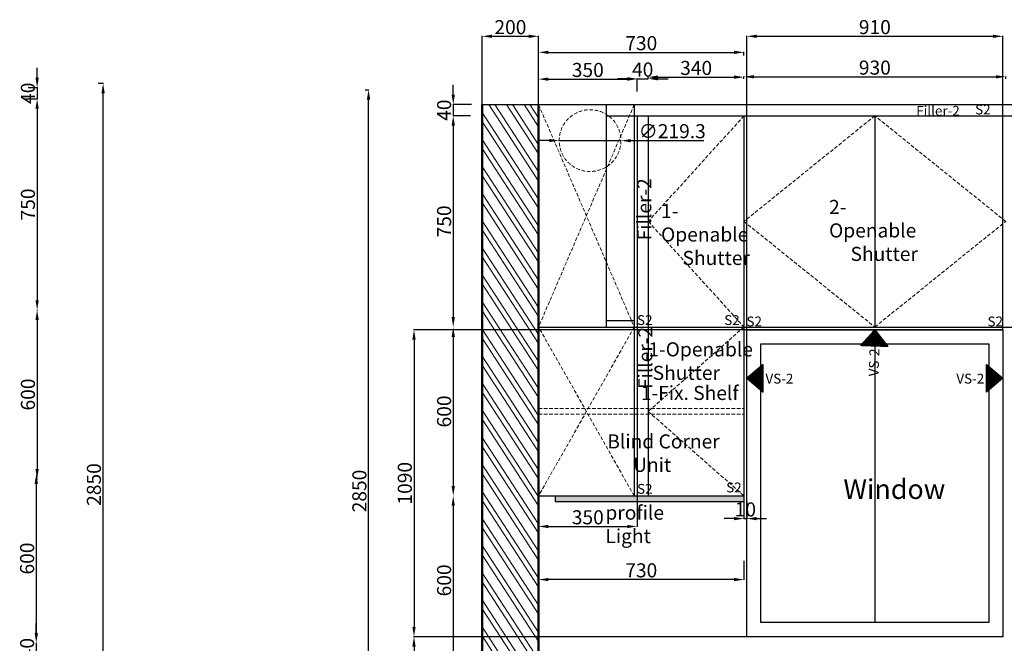
# Model space of a CAD drawing. Units: millimetres. Extents: x 407065 to 421840, y 1168257 to 1177792.
# Tile 16 of 17: x 415758 to 419256, y 1175003 to 1177218. Entities that reach past the tile are written whole.
import ezdxf

# ---------------------------------------------------------------- set-up
doc = ezdxf.new("R2010")
doc.units = ezdxf.units.MM
doc.linetypes.add('DASHED', pattern=[19.05, 12.7, -6.35])
for name, color, linetype, lineweight in [('A-ANNO-DIMS', 6, 'Continuous', 18), ('A-ANNO-TEXT', 30, 'Continuous', 18), ('A-FURN', 3, 'Continuous', 25), ('A-FURN-HIDN', 7, 'DASHED', 18), ('A-FURN-PATT', 252, 'Continuous', 13), ('A-GLAZ', 4, 'Continuous', 25), ('A-WALL', 7, 'Continuous', 50), ('A-WALL-PATT', 8, 'Continuous', 13)]:
    doc.layers.add(name, color=color, linetype=linetype, lineweight=lineweight)
doc.styles.get("Standard").update_dxf_attribs({"font": 'arial.ttf'})
doc.dimstyles.new('ISO-25', dxfattribs={"dimtxt": 50, "dimasz": 35, "dimexe": 1.25, "dimexo": 0.625, "dimtad": 1, "dimdec": 1, "dimtxsty": 'Standard', "dimcen": 35, "dimadec": 0, "dimazin": 0, "dimtfac": 1, "dimtdec": 1, "dimtmove": 0, "dimatfit": 3, "dimfxl": 1, "dimarcsym": 0})

# ---------------------------------------------------------------- blocks, each defined once
blk = doc.blocks.new('*D63')
at = {"layer": 'A-ANNO-DIMS', "color": 0, "lineweight": -2, "transparency": 16777216}
for p, q in [((415819.6, 1177011.4), (415819.6, 1177046.4)), ((415788, 1176976.4), (415820.8, 1176976.4)), ((415819.6, 1176976.4), (415819.6, 1176936.4)), ((415777.3, 1176936.4), (415820.8, 1176936.4)), ((415819.6, 1176901.4), (415819.6, 1176866.4))]:
    blk.add_line(p, q, dxfattribs=at)
at = {"layer": 'A-ANNO-DIMS', "color": 0, "transparency": 16777216}
for points in [[(415813.7, 1177011.4), (415825.4, 1177011.4), (415819.6, 1176976.4)], [(415813.7, 1176901.4), (415825.4, 1176901.4), (415819.6, 1176936.4)]]:
    blk.add_solid(points, dxfattribs=at)
at = {"layer": 'Defpoints', "color": 0, "transparency": 16777216}
for p in [(415787.4, 1176976.4), (415776.6, 1176936.4), (415819.6, 1176936.4)]:
    blk.add_point(p, dxfattribs=at)
at = {"layer": 'A-ANNO-DIMS', "color": 0, "transparency": 16777216, "insert": (415793.4, 1176956.4), "char_height": 50, "attachment_point": 5, "rotation": 90}
blk.add_mtext('40', dxfattribs=at)
blk = doc.blocks.new('*D64')
at = {"layer": 'A-ANNO-DIMS', "color": 0, "lineweight": -2, "transparency": 16777216}
for p, q in [((415820.2, 1176936.4), (415820.8, 1176936.4)), ((415819.6, 1176901.4), (415819.6, 1176221.4)), ((415820.2, 1176186.4), (415820.8, 1176186.4))]:
    blk.add_line(p, q, dxfattribs=at)
at = {"layer": 'A-ANNO-DIMS', "color": 0, "transparency": 16777216}
for points in [[(415813.7, 1176901.4), (415825.4, 1176901.4), (415819.6, 1176936.4)], [(415813.7, 1176221.4), (415825.4, 1176221.4), (415819.6, 1176186.4)]]:
    blk.add_solid(points, dxfattribs=at)
at = {"layer": 'Defpoints', "color": 0, "transparency": 16777216}
for p in [(415819.6, 1176936.4), (415819.6, 1176186.4), (415819.6, 1176186.4)]:
    blk.add_point(p, dxfattribs=at)
at = {"layer": 'A-ANNO-DIMS', "color": 0, "transparency": 16777216, "insert": (415793.4, 1176561.4), "char_height": 50, "attachment_point": 5, "rotation": 90}
blk.add_mtext('750', dxfattribs=at)
blk = doc.blocks.new('*D65')
at = {"layer": 'A-ANNO-DIMS', "color": 0, "lineweight": -2, "transparency": 16777216}
for p, q in [((415818.9, 1176186.4), (415820.8, 1176186.4)), ((415819.6, 1176151.4), (415819.6, 1175621.4)), ((415818.9, 1175586.4), (415820.8, 1175586.4))]:
    blk.add_line(p, q, dxfattribs=at)
at = {"layer": 'A-ANNO-DIMS', "color": 0, "transparency": 16777216}
for points in [[(415813.7, 1176151.4), (415825.4, 1176151.4), (415819.6, 1176186.4)], [(415813.7, 1175621.4), (415825.4, 1175621.4), (415819.6, 1175586.4)]]:
    blk.add_solid(points, dxfattribs=at)
at = {"layer": 'Defpoints', "color": 0, "transparency": 16777216}
for p in [(415818.3, 1176186.4), (415818.3, 1175586.4), (415819.6, 1175586.4)]:
    blk.add_point(p, dxfattribs=at)
at = {"layer": 'A-ANNO-DIMS', "color": 0, "transparency": 16777216, "insert": (415793.4, 1175886.4), "char_height": 50, "attachment_point": 5, "rotation": 90}
blk.add_mtext('600', dxfattribs=at)
blk = doc.blocks.new('*D66')
at = {"layer": 'A-ANNO-DIMS', "color": 0, "lineweight": -2, "transparency": 16777216}
for p, q in [((415817.3, 1175603.9), (415817.9, 1175603.9)), ((415816.7, 1175568.9), (415816.7, 1175038.9)), ((415817.3, 1175003.9), (415817.9, 1175003.9))]:
    blk.add_line(p, q, dxfattribs=at)
at = {"layer": 'A-ANNO-DIMS', "color": 0, "transparency": 16777216}
for points in [[(415810.8, 1175568.9), (415822.5, 1175568.9), (415816.7, 1175603.9)], [(415810.8, 1175038.9), (415822.5, 1175038.9), (415816.7, 1175003.9)]]:
    blk.add_solid(points, dxfattribs=at)
at = {"layer": 'Defpoints', "color": 0, "transparency": 16777216}
for p in [(415816.7, 1175603.9), (415816.7, 1175003.9), (415816.7, 1175003.9)]:
    blk.add_point(p, dxfattribs=at)
at = {"layer": 'A-ANNO-DIMS', "color": 0, "transparency": 16777216, "insert": (415790.5, 1175303.9), "char_height": 50, "attachment_point": 5, "rotation": 90}
blk.add_mtext('600', dxfattribs=at)
blk = doc.blocks.new('*D67')
at = {"layer": 'A-ANNO-DIMS', "color": 0, "lineweight": -2, "transparency": 16777216}
for p, q in [((415816.7, 1175038.9), (415816.7, 1175073.9)), ((415816.7, 1175003.9), (415816.7, 1174963.9)), ((415817.3, 1175003.9), (415817.9, 1175003.9)), ((415817.3, 1174963.9), (415817.9, 1174963.9)), ((415816.7, 1174928.9), (415816.7, 1174893.9))]:
    blk.add_line(p, q, dxfattribs=at)
at = {"layer": 'A-ANNO-DIMS', "color": 0, "transparency": 16777216}
for points in [[(415810.8, 1175038.9), (415822.5, 1175038.9), (415816.7, 1175003.9)], [(415810.8, 1174928.9), (415822.5, 1174928.9), (415816.7, 1174963.9)]]:
    blk.add_solid(points, dxfattribs=at)
at = {"layer": 'Defpoints', "color": 0, "transparency": 16777216}
for p in [(415816.7, 1175003.9), (415816.7, 1174963.9), (415816.7, 1174963.9)]:
    blk.add_point(p, dxfattribs=at)
at = {"layer": 'A-ANNO-DIMS', "color": 0, "transparency": 16777216, "insert": (415790.5, 1174983.9), "char_height": 50, "attachment_point": 5, "rotation": 90}
blk.add_mtext('40', dxfattribs=at)
blk = doc.blocks.new('*D71')
at = {"layer": 'A-ANNO-DIMS', "color": 0, "lineweight": -2, "transparency": 16777216}
for p, q in [((416036.8, 1176991.7), (416055.3, 1176991.7)), ((416054.1, 1174176.7), (416054.1, 1176956.7)), ((416036.8, 1174141.7), (416055.3, 1174141.7))]:
    blk.add_line(p, q, dxfattribs=at)
at = {"layer": 'A-ANNO-DIMS', "color": 0, "transparency": 16777216}
for points in [[(416048.2, 1176956.7), (416059.9, 1176956.7), (416054.1, 1176991.7)], [(416048.2, 1174176.7), (416059.9, 1174176.7), (416054.1, 1174141.7)]]:
    blk.add_solid(points, dxfattribs=at)
at = {"layer": 'Defpoints', "color": 0, "transparency": 16777216}
for p in [(416036.2, 1176991.7), (416054.1, 1176991.7), (416036.2, 1174141.7)]:
    blk.add_point(p, dxfattribs=at)
at = {"layer": 'A-ANNO-DIMS', "color": 0, "transparency": 16777216, "insert": (416027.9, 1175566.7), "char_height": 50, "attachment_point": 5, "rotation": 90}
blk.add_mtext('2850', dxfattribs=at)
blk = doc.blocks.new('*D82')
at = {"layer": 'A-ANNO-DIMS', "color": 0, "lineweight": -2, "transparency": 16777216}
for p, q in [((417601.3, 1176962.9), (417601.3, 1177007.8)), ((417636.3, 1177006.6), (417916.3, 1177006.6)), ((417951.3, 1176962.9), (417951.3, 1177007.8))]:
    blk.add_line(p, q, dxfattribs=at)
at = {"layer": 'A-ANNO-DIMS', "color": 0, "transparency": 16777216}
for points in [[(417636.3, 1177012.4), (417636.3, 1177000.7), (417601.3, 1177006.6)], [(417916.3, 1177012.4), (417916.3, 1177000.7), (417951.3, 1177006.6)]]:
    blk.add_solid(points, dxfattribs=at)
at = {"layer": 'Defpoints', "color": 0, "transparency": 16777216}
for p in [(417951.3, 1177006.6), (417601.3, 1176962.3), (417951.3, 1176962.3)]:
    blk.add_point(p, dxfattribs=at)
at = {"layer": 'A-ANNO-DIMS', "color": 0, "transparency": 16777216, "insert": (417776.3, 1177032.7), "char_height": 50, "attachment_point": 5}
blk.add_mtext('350', dxfattribs=at)
blk = doc.blocks.new('*D83')
at = {"layer": 'A-ANNO-DIMS', "color": 0, "lineweight": -2, "transparency": 16777216}
for p, q in [((417916.3, 1177007.8), (417881.3, 1177007.8)), ((417951.3, 1177007.2), (417951.3, 1177009.1)), ((417951.3, 1177007.8), (417991.3, 1177007.8)), ((417991.3, 1177007.2), (417991.3, 1177009.1)), ((418026.3, 1177007.8), (418061.3, 1177007.8))]:
    blk.add_line(p, q, dxfattribs=at)
at = {"layer": 'A-ANNO-DIMS', "color": 0, "transparency": 16777216}
for points in [[(417916.3, 1177013.7), (417916.3, 1177002), (417951.3, 1177007.8)], [(418026.3, 1177013.7), (418026.3, 1177002), (417991.3, 1177007.8)]]:
    blk.add_solid(points, dxfattribs=at)
at = {"layer": 'Defpoints', "color": 0, "transparency": 16777216}
for p in [(417951.3, 1177006.6), (417991.3, 1177007.8), (417991.3, 1177006.6)]:
    blk.add_point(p, dxfattribs=at)
at = {"layer": 'A-ANNO-DIMS', "color": 0, "transparency": 16777216, "insert": (417971.3, 1177034), "char_height": 50, "attachment_point": 5}
blk.add_mtext('40', dxfattribs=at)
blk = doc.blocks.new('*D84')
at = {"layer": 'A-ANNO-DIMS', "color": 0, "lineweight": -2, "transparency": 16777216}
for p, q in [((417991.3, 1177007.2), (417991.3, 1177014.9)), ((418026.3, 1177013.6), (418296.3, 1177013.6)), ((418331.3, 1177007.2), (418331.3, 1177014.9))]:
    blk.add_line(p, q, dxfattribs=at)
at = {"layer": 'A-ANNO-DIMS', "color": 0, "transparency": 16777216}
for points in [[(418026.3, 1177019.5), (418026.3, 1177007.8), (417991.3, 1177013.6)], [(418296.3, 1177019.5), (418296.3, 1177007.8), (418331.3, 1177013.6)]]:
    blk.add_solid(points, dxfattribs=at)
at = {"layer": 'Defpoints', "color": 0, "transparency": 16777216}
for p in [(417991.3, 1177006.6), (418331.3, 1177013.6), (418331.3, 1177006.6)]:
    blk.add_point(p, dxfattribs=at)
at = {"layer": 'A-ANNO-DIMS', "color": 0, "transparency": 16777216, "insert": (418161.3, 1177039.8), "char_height": 50, "attachment_point": 5}
blk.add_mtext('340', dxfattribs=at)
blk = doc.blocks.new('*D85')
at = {"layer": 'A-ANNO-DIMS', "color": 0, "lineweight": -2, "transparency": 16777216}
for p, q in [((417601.3, 1177090.2), (417601.3, 1177103)), ((417636.3, 1177101.7), (418296.3, 1177101.7)), ((418331.3, 1177090.2), (418331.3, 1177103))]:
    blk.add_line(p, q, dxfattribs=at)
at = {"layer": 'A-ANNO-DIMS', "color": 0, "transparency": 16777216}
for points in [[(417636.3, 1177107.6), (417636.3, 1177095.9), (417601.3, 1177101.7)], [(418296.3, 1177107.6), (418296.3, 1177095.9), (418331.3, 1177101.7)]]:
    blk.add_solid(points, dxfattribs=at)
at = {"layer": 'Defpoints', "color": 0, "transparency": 16777216}
for p in [(418331.3, 1177101.7), (417601.3, 1177089.6), (418331.3, 1177089.6)]:
    blk.add_point(p, dxfattribs=at)
at = {"layer": 'A-ANNO-DIMS', "color": 0, "transparency": 16777216, "insert": (417966.3, 1177127.9), "char_height": 50, "attachment_point": 5}
blk.add_mtext('730', dxfattribs=at)
blk = doc.blocks.new('*D86')
at = {"layer": 'A-ANNO-DIMS', "color": 0, "lineweight": -2, "transparency": 16777216}
for p, q in [((418331.3, 1177007.2), (418331.3, 1177016.1)), ((418366.3, 1177014.9), (419226.3, 1177014.9)), ((419261.3, 1177007.2), (419261.3, 1177016.1))]:
    blk.add_line(p, q, dxfattribs=at)
at = {"layer": 'A-ANNO-DIMS', "color": 0, "transparency": 16777216}
for points in [[(418366.3, 1177020.7), (418366.3, 1177009), (418331.3, 1177014.9)], [(419226.3, 1177020.7), (419226.3, 1177009), (419261.3, 1177014.9)]]:
    blk.add_solid(points, dxfattribs=at)
at = {"layer": 'Defpoints', "color": 0, "transparency": 16777216}
for p in [(418331.3, 1177006.6), (419261.3, 1177014.9), (419261.3, 1177006.6)]:
    blk.add_point(p, dxfattribs=at)
at = {"layer": 'A-ANNO-DIMS', "color": 0, "transparency": 16777216, "insert": (418796.3, 1177041), "char_height": 50, "attachment_point": 5}
blk.add_mtext('930', dxfattribs=at)
blk = doc.blocks.new('*D104')
at = {"layer": 'A-ANNO-DIMS', "color": 0, "lineweight": -2, "transparency": 16777216}
for p, q in [((417298.2, 1176951.2), (417298.2, 1176986.2)), ((417362.5, 1176916.2), (417297, 1176916.2)), ((417298.2, 1176916.2), (417298.2, 1176876.2)), ((417359.5, 1176876.2), (417297, 1176876.2)), ((417298.2, 1176841.2), (417298.2, 1176806.2))]:
    blk.add_line(p, q, dxfattribs=at)
at = {"layer": 'A-ANNO-DIMS', "color": 0, "transparency": 16777216}
for points in [[(417292.4, 1176951.2), (417304, 1176951.2), (417298.2, 1176916.2)], [(417292.4, 1176841.2), (417304, 1176841.2), (417298.2, 1176876.2)]]:
    blk.add_solid(points, dxfattribs=at)
at = {"layer": 'Defpoints', "color": 0, "transparency": 16777216}
for p in [(417363.1, 1176916.2), (417298.2, 1176876.2), (417360.1, 1176876.2)]:
    blk.add_point(p, dxfattribs=at)
at = {"layer": 'A-ANNO-DIMS', "color": 0, "transparency": 16777216, "insert": (417272.1, 1176896.2), "char_height": 50, "attachment_point": 5, "rotation": 90}
blk.add_mtext('40', dxfattribs=at)
blk = doc.blocks.new('*D105')
at = {"layer": 'A-ANNO-DIMS', "color": 0, "lineweight": -2, "transparency": 16777216}
for p, q in [((417298.8, 1176876.2), (417299.5, 1176876.2)), ((417298.2, 1176841.2), (417298.2, 1176161.2)), ((417298.8, 1176126.2), (417299.5, 1176126.2))]:
    blk.add_line(p, q, dxfattribs=at)
at = {"layer": 'A-ANNO-DIMS', "color": 0, "transparency": 16777216}
for points in [[(417292.4, 1176841.2), (417304, 1176841.2), (417298.2, 1176876.2)], [(417292.4, 1176161.2), (417304, 1176161.2), (417298.2, 1176126.2)]]:
    blk.add_solid(points, dxfattribs=at)
at = {"layer": 'Defpoints', "color": 0, "transparency": 16777216}
for p in [(417298.2, 1176876.2), (417298.2, 1176126.2), (417298.2, 1176126.2)]:
    blk.add_point(p, dxfattribs=at)
at = {"layer": 'A-ANNO-DIMS', "color": 0, "transparency": 16777216, "insert": (417272.1, 1176501.2), "char_height": 50, "attachment_point": 5, "rotation": 90}
blk.add_mtext('750', dxfattribs=at)
blk = doc.blocks.new('*D106')
at = {"layer": 'A-ANNO-DIMS', "color": 0, "lineweight": -2, "transparency": 16777216}
for p, q in [((417298.8, 1176126.2), (417299.5, 1176126.2)), ((417298.2, 1176091.2), (417298.2, 1175561.2)), ((417298.8, 1175526.2), (417299.5, 1175526.2))]:
    blk.add_line(p, q, dxfattribs=at)
at = {"layer": 'A-ANNO-DIMS', "color": 0, "transparency": 16777216}
for points in [[(417292.4, 1176091.2), (417304, 1176091.2), (417298.2, 1176126.2)], [(417292.4, 1175561.2), (417304, 1175561.2), (417298.2, 1175526.2)]]:
    blk.add_solid(points, dxfattribs=at)
at = {"layer": 'Defpoints', "color": 0, "transparency": 16777216}
for p in [(417298.2, 1176126.2), (417298.2, 1175526.2), (417298.2, 1175526.2)]:
    blk.add_point(p, dxfattribs=at)
at = {"layer": 'A-ANNO-DIMS', "color": 0, "transparency": 16777216, "insert": (417272.1, 1175826.2), "char_height": 50, "attachment_point": 5, "rotation": 90}
blk.add_mtext('600', dxfattribs=at)
blk = doc.blocks.new('*D107')
at = {"layer": 'A-ANNO-DIMS', "color": 0, "lineweight": -2, "transparency": 16777216}
for p, q in [((417298.8, 1175526.2), (417299.5, 1175526.2)), ((417298.2, 1175491.2), (417298.2, 1174961.2)), ((417298.8, 1174926.2), (417299.5, 1174926.2))]:
    blk.add_line(p, q, dxfattribs=at)
at = {"layer": 'A-ANNO-DIMS', "color": 0, "transparency": 16777216}
for points in [[(417292.4, 1175491.2), (417304, 1175491.2), (417298.2, 1175526.2)], [(417292.4, 1174961.2), (417304, 1174961.2), (417298.2, 1174926.2)]]:
    blk.add_solid(points, dxfattribs=at)
at = {"layer": 'Defpoints', "color": 0, "transparency": 16777216}
for p in [(417298.2, 1175526.2), (417298.2, 1174926.2), (417298.2, 1174926.2)]:
    blk.add_point(p, dxfattribs=at)
at = {"layer": 'A-ANNO-DIMS', "color": 0, "transparency": 16777216, "insert": (417272.1, 1175226.2), "char_height": 50, "attachment_point": 5, "rotation": 90}
blk.add_mtext('600', dxfattribs=at)
blk = doc.blocks.new('*D112')
at = {"layer": 'A-ANNO-DIMS', "color": 0, "lineweight": -2, "transparency": 16777216}
for p, q in [((416985.7, 1176968.7), (416998.5, 1176968.7)), ((416997.3, 1174153.7), (416997.3, 1176933.7)), ((416985.7, 1174118.7), (416998.5, 1174118.7))]:
    blk.add_line(p, q, dxfattribs=at)
at = {"layer": 'A-ANNO-DIMS', "color": 0, "transparency": 16777216}
for points in [[(416991.4, 1176933.7), (417003.1, 1176933.7), (416997.3, 1176968.7)], [(416991.4, 1174153.7), (417003.1, 1174153.7), (416997.3, 1174118.7)]]:
    blk.add_solid(points, dxfattribs=at)
at = {"layer": 'Defpoints', "color": 0, "transparency": 16777216}
for p in [(416985.1, 1176968.7), (416997.3, 1176968.7), (416985.1, 1174118.7)]:
    blk.add_point(p, dxfattribs=at)
at = {"layer": 'A-ANNO-DIMS', "color": 0, "transparency": 16777216, "insert": (416971.1, 1175543.7), "char_height": 50, "attachment_point": 5, "rotation": 90}
blk.add_mtext('2850', dxfattribs=at)
blk = doc.blocks.new('*D113')
at = {"layer": 'A-ANNO-DIMS', "color": 0, "lineweight": -2, "transparency": 16777216}
for p, q in [((417601.3, 1175525.5), (417601.3, 1175416.4)), ((417951.3, 1175525.5), (417951.3, 1175416.4)), ((417636.3, 1175417.7), (417916.3, 1175417.7))]:
    blk.add_line(p, q, dxfattribs=at)
at = {"layer": 'A-ANNO-DIMS', "color": 0, "transparency": 16777216}
for points in [[(417636.3, 1175423.5), (417636.3, 1175411.8), (417601.3, 1175417.7)], [(417916.3, 1175423.5), (417916.3, 1175411.8), (417951.3, 1175417.7)]]:
    blk.add_solid(points, dxfattribs=at)
at = {"layer": 'Defpoints', "color": 0, "transparency": 16777216}
for p in [(417601.3, 1175526.2), (417951.3, 1175526.2), (417951.3, 1175417.7)]:
    blk.add_point(p, dxfattribs=at)
at = {"layer": 'A-ANNO-DIMS', "color": 0, "transparency": 16777216, "insert": (417776.3, 1175443.8), "char_height": 50, "attachment_point": 5}
blk.add_mtext('350', dxfattribs=at)
blk = doc.blocks.new('*D114')
at = {"layer": 'A-ANNO-DIMS', "color": 0, "lineweight": -2, "transparency": 16777216}
for p, q in [((418331.3, 1175505.5), (418331.3, 1175444.4)), ((418341.3, 1175505.5), (418341.3, 1175444.4)), ((418296.3, 1175445.6), (418261.3, 1175445.6)), ((418331.3, 1175445.6), (418341.3, 1175445.6)), ((418376.3, 1175445.6), (418411.3, 1175445.6))]:
    blk.add_line(p, q, dxfattribs=at)
at = {"layer": 'A-ANNO-DIMS', "color": 0, "transparency": 16777216}
for points in [[(418296.3, 1175451.5), (418296.3, 1175439.8), (418331.3, 1175445.6)], [(418376.3, 1175451.5), (418376.3, 1175439.8), (418341.3, 1175445.6)]]:
    blk.add_solid(points, dxfattribs=at)
at = {"layer": 'Defpoints', "color": 0, "transparency": 16777216}
for p in [(418331.3, 1175506.2), (418341.3, 1175506.2), (418341.3, 1175445.6)]:
    blk.add_point(p, dxfattribs=at)
at = {"layer": 'A-ANNO-DIMS', "color": 0, "transparency": 16777216, "insert": (418336.3, 1175471.8), "char_height": 50, "attachment_point": 5}
blk.add_mtext('10', dxfattribs=at)
blk = doc.blocks.new('*D115')
at = {"layer": 'A-ANNO-DIMS', "color": 0, "lineweight": -2, "transparency": 16777216}
for p, q in [((418331.3, 1175295.9), (418331.3, 1175227.9)), ((417601.3, 1175276), (417601.3, 1175227.9)), ((418296.3, 1175229.2), (417636.3, 1175229.2))]:
    blk.add_line(p, q, dxfattribs=at)
at = {"layer": 'A-ANNO-DIMS', "color": 0, "transparency": 16777216}
for points in [[(417636.3, 1175235), (417636.3, 1175223.4), (417601.3, 1175229.2)], [(418296.3, 1175235), (418296.3, 1175223.4), (418331.3, 1175229.2)]]:
    blk.add_solid(points, dxfattribs=at)
at = {"layer": 'Defpoints', "color": 0, "transparency": 16777216}
for p in [(418331.3, 1175296.5), (417601.3, 1175276.6), (417601.3, 1175229.2)]:
    blk.add_point(p, dxfattribs=at)
at = {"layer": 'A-ANNO-DIMS', "color": 0, "transparency": 16777216, "insert": (417966.3, 1175255.4), "char_height": 50, "attachment_point": 5}
blk.add_mtext('730', dxfattribs=at)
blk = doc.blocks.new('SHUTTER-HANDLE-MARK')
h = blk.add_hatch()
h.set_pattern_fill('ANSI32', color=256, scale=0.08)
h.set_pattern_definition([(45, (-3404.92366, -221.627), (-0.53881536726, 0.53881536726), []), (45, (-3404.56445, -221.627), (-0.53881536726, 0.53881536726), [])])
h.paths.add_polyline_path([(420059.2, 1176549.9), (420001.3, 1176501.2), (420059.2, 1176452.5)])
h = blk.add_hatch(color=256)
h.dxf.hatch_style = 1
h.paths.add_polyline_path([(420059.2, 1176549.9), (420001.3, 1176501.2), (420059.2, 1176452.5)])
blk = doc.blocks.new('*D201')
at = {"layer": 'A-ANNO-DIMS', "color": 0, "lineweight": -2, "transparency": 16777216}
for p, q in [((417401.3, 1176916.8), (417401.3, 1177159.9)), ((417436.3, 1177158.7), (417566.3, 1177158.7)), ((417601.3, 1176916.8), (417601.3, 1177159.9))]:
    blk.add_line(p, q, dxfattribs=at)
at = {"layer": 'A-ANNO-DIMS', "color": 0, "transparency": 16777216}
for points in [[(417436.3, 1177164.5), (417436.3, 1177152.8), (417401.3, 1177158.7)], [(417566.3, 1177164.5), (417566.3, 1177152.8), (417601.3, 1177158.7)]]:
    blk.add_solid(points, dxfattribs=at)
at = {"layer": 'Defpoints', "color": 0, "transparency": 16777216}
for p in [(417601.3, 1177158.7), (417401.3, 1176916.2), (417601.3, 1176916.2)]:
    blk.add_point(p, dxfattribs=at)
at = {"layer": 'A-ANNO-DIMS', "color": 0, "transparency": 16777216, "insert": (417501.3, 1177184.8), "char_height": 50, "attachment_point": 5}
blk.add_mtext('200', dxfattribs=at)
blk = doc.blocks.new('*D203')
at = {"layer": 'A-ANNO-DIMS', "color": 0, "lineweight": -2, "transparency": 16777216}
for p, q in [((418340.7, 1175026.2), (417157.5, 1175026.2)), ((417158.8, 1174991.2), (417158.8, 1174101.2)), ((417600.7, 1174066.2), (417157.5, 1174066.2))]:
    blk.add_line(p, q, dxfattribs=at)
at = {"layer": 'A-ANNO-DIMS', "color": 0, "transparency": 16777216}
for points in [[(417152.9, 1174991.2), (417164.6, 1174991.2), (417158.8, 1175026.2)], [(417152.9, 1174101.2), (417164.6, 1174101.2), (417158.8, 1174066.2)]]:
    blk.add_solid(points, dxfattribs=at)
at = {"layer": 'Defpoints', "color": 0, "transparency": 16777216}
for p in [(418341.3, 1175026.2), (417158.8, 1174066.2), (417601.3, 1174066.2)]:
    blk.add_point(p, dxfattribs=at)
at = {"layer": 'A-ANNO-DIMS', "color": 0, "transparency": 16777216, "insert": (417132.6, 1174546.2), "char_height": 50, "attachment_point": 5, "rotation": 90}
blk.add_mtext('960', dxfattribs=at)
blk = doc.blocks.new('*D204')
at = {"layer": 'A-ANNO-DIMS', "color": 0, "lineweight": -2, "transparency": 16777216}
for p, q in [((419250.7, 1176116.2), (417157.5, 1176116.2)), ((417158.8, 1176081.2), (417158.8, 1175061.2)), ((419250.7, 1175026.2), (417157.5, 1175026.2))]:
    blk.add_line(p, q, dxfattribs=at)
at = {"layer": 'A-ANNO-DIMS', "color": 0, "transparency": 16777216}
for points in [[(417152.9, 1176081.2), (417164.6, 1176081.2), (417158.8, 1176116.2)], [(417152.9, 1175061.2), (417164.6, 1175061.2), (417158.8, 1175026.2)]]:
    blk.add_solid(points, dxfattribs=at)
at = {"layer": 'Defpoints', "color": 0, "transparency": 16777216}
for p in [(419251.3, 1176116.2), (417158.8, 1175026.2), (419251.3, 1175026.2)]:
    blk.add_point(p, dxfattribs=at)
at = {"layer": 'A-ANNO-DIMS', "color": 0, "transparency": 16777216, "insert": (417132.6, 1175571.2), "char_height": 50, "attachment_point": 5, "rotation": 90}
blk.add_mtext('1090', dxfattribs=at)
blk = doc.blocks.new('*D205')
at = {"layer": 'A-ANNO-DIMS', "color": 0, "lineweight": -2, "transparency": 16777216}
for p, q in [((418341.3, 1176116.8), (418341.3, 1177159.9)), ((418376.3, 1177158.7), (419216.3, 1177158.7)), ((419251.3, 1176116.8), (419251.3, 1177159.9))]:
    blk.add_line(p, q, dxfattribs=at)
at = {"layer": 'A-ANNO-DIMS', "color": 0, "transparency": 16777216}
for points in [[(418376.3, 1177164.5), (418376.3, 1177152.8), (418341.3, 1177158.7)], [(419216.3, 1177164.5), (419216.3, 1177152.8), (419251.3, 1177158.7)]]:
    blk.add_solid(points, dxfattribs=at)
at = {"layer": 'Defpoints', "color": 0, "transparency": 16777216}
for p in [(419251.3, 1177158.7), (418341.3, 1176116.2), (419251.3, 1176116.2)]:
    blk.add_point(p, dxfattribs=at)
at = {"layer": 'A-ANNO-DIMS', "color": 0, "transparency": 16777216, "insert": (418796.3, 1177184.8), "char_height": 50, "attachment_point": 5}
blk.add_mtext('910', dxfattribs=at)
blk = doc.blocks.new('*D239')
at = {"layer": 'A-ANNO-DIMS', "color": 0, "lineweight": -2, "transparency": 16777216}
for p, q in [((417639.7, 1176788.4), (417604.7, 1176788.5)), ((417674.7, 1176788.4), (417894, 1176788)), ((418188.4, 1176787.5), (417929, 1176787.9))]:
    blk.add_line(p, q, dxfattribs=at)
at = {"layer": 'A-ANNO-DIMS', "color": 0, "transparency": 16777216}
for points in [[(417639.7, 1176794.3), (417639.7, 1176782.6), (417674.7, 1176788.4)], [(417929, 1176793.8), (417929, 1176782.1), (417894, 1176788)]]:
    blk.add_solid(points, dxfattribs=at)
at = {"layer": 'Defpoints', "color": 0, "transparency": 16777216}
for p in [(417674.7, 1176788.4), (417894, 1176788)]:
    blk.add_point(p, dxfattribs=at)
at = {"layer": 'A-ANNO-DIMS', "color": 0, "transparency": 16777216, "insert": (418076.2, 1176815.2), "char_height": 50, "attachment_point": 5, "rotation": 359.8986}
blk.add_mtext('∅219.3', dxfattribs=at)

msp = doc.modelspace()

# ---------------------------------------------------------------- hatches: boundary and pattern name
at = {"layer": 'A-FURN-PATT'}
h = msp.add_hatch(color=256, dxfattribs=at)
h.dxf.hatch_style = 1
h.paths.add_polyline_path([(418331.277, 1175526.1682), (417660.9056, 1175526.1682), (417660.9056, 1175506.1682), (418331.277, 1175506.1682)])
at = {"layer": 'A-WALL-PATT'}
h = msp.add_hatch(dxfattribs=at)
h.set_pattern_fill('ANSI32', color=256, scale=5.5, angle=78)
h.set_pattern_definition([(123, (-3404.924, -221.627), (-43.9358544, -28.5322774), []), (123, (-3399.79, -197.47), (-43.9358544, -28.5322774), [])])
h.paths.add_polyline_path([(417601.277, 1176916.1682), (417401.277, 1176916.1682), (417401.277, 1174066.1682), (417601.277, 1174066.1682)])

# ---------------------------------------------------------------- linework, layer by layer
at = {"layer": 'A-FURN'}
for p, q in [((417401.277, 1176916.1682), (421591.277, 1176916.1682)), ((417841.277, 1176916.1682), (417841.277, 1176126.1682)), ((417941.277, 1176916.1682), (417941.277, 1175526.1682)), ((417841.277, 1176876.1682), (420001.277, 1176876.1682)), ((417951.277, 1176876.1682), (417951.277, 1175526.1682)), ((417991.277, 1176876.1682), (417991.277, 1175526.1682)), ((418331.277, 1176876.1682), (418331.277, 1175506.1682)), ((418796.277, 1176876.1682), (418796.277, 1176126.1682)), ((417601.277, 1176126.1682), (420001.277, 1176126.1682)), ((417841.277, 1176149.1114), (417941.277, 1176149.1114)), ((417601.277, 1175526.1682), (418331.277, 1175526.1682)), ((417660.9056, 1175526.1682), (417660.9056, 1175506.1682)), ((417660.9056, 1175506.1682), (418331.277, 1175506.1682))]:
    msp.add_line(p, q, dxfattribs=at)
at = {"layer": 'A-FURN-HIDN'}
for p, q in [((417601.277, 1176916.1682), (417941.277, 1176126.1682)), ((417941.277, 1176916.1682), (417601.277, 1176126.1682)), ((418796.277, 1176876.1682), (418331.277, 1176501.1682)), ((419261.277, 1176501.1682), (418796.277, 1176876.1682)), ((418331.277, 1176501.1682), (418796.277, 1176126.1682)), ((418796.277, 1176126.1682), (419261.277, 1176501.1682)), ((417941.277, 1175526.1682), (417601.277, 1176126.1682)), ((417941.277, 1176126.1682), (417601.277, 1175526.1682)), ((417601.277, 1175836.1682), (418331.277, 1175836.1682)), ((417601.277, 1175816.1682), (418331.277, 1175816.1682))]:
    msp.add_line(p, q, dxfattribs=at)
msp.add_lwpolyline([(418331.277, 1176876.1682), (417991.277, 1176501.1682), (418331.277, 1176126.1682), (417991.277, 1175826.13), (418331.277, 1175526.1682)], dxfattribs=at)
msp.add_circle((417784.3431, 1176788.1923), 109.6486, dxfattribs=at)
at = {"layer": 'A-GLAZ'}
msp.add_line((418796.277, 1176066.1682), (418796.277, 1175076.1682), dxfattribs=at)
msp.add_lwpolyline([(419251.277, 1175026.1682), (418341.277, 1175026.1682), (418341.277, 1176116.1682), (419251.277, 1176116.1682), (419251.277, 1175026.1682)], dxfattribs=at)
for points in [[(418745.6063, 1176059.9751), (418796.277, 1176116.1682), (418842.9149, 1176056.5855)], [(419201.277, 1175076.1682), (418391.277, 1175076.1682), (418391.277, 1176066.1682), (419201.277, 1176066.1682)], [(418399.2, 1175992.5585), (418341.277, 1175943.8747), (418399.2, 1175895.1909)], [(419193.354, 1175992.5585), (419251.277, 1175943.8747), (419193.354, 1175895.1909)]]:
    msp.add_lwpolyline(points, close=True, dxfattribs=at)
at = {"layer": 'A-WALL'}
for p, q in [((417401.277, 1176916.1682), (417401.277, 1174066.1682)), ((417601.277, 1176916.1682), (417601.277, 1174066.1682))]:
    msp.add_line(p, q, dxfattribs=at)

# ---------------------------------------------------------------- block references
at = {"layer": 'A-FURN', "extrusion": (0, 0, -1), "zscale": -1, "rotation": 271.9949857405152}
msp.add_blockref('SHUTTER-HANDLE-MARK', (-1609205.4403, 1554906.4737), dxfattribs=at)
at = {"layer": 'A-FURN'}
msp.add_blockref('SHUTTER-HANDLE-MARK', (-1660, -557.2935), dxfattribs=at)
at = {"layer": 'A-FURN', "extrusion": (0, 0, -1), "zscale": -1}
msp.add_blockref('SHUTTER-HANDLE-MARK', (-839252.554, -557.2935), dxfattribs=at)

# ---------------------------------------------------------------- texts
at = {"layer": 'A-ANNO-TEXT'}
for s, width, insert, char_height, attachment_point in [('     Filler-2', 382.409863, (418889.8195, 1176911.483), 35, 1), ('S2', 382.409863, (419152.5855, 1176916.1682), 35, 1), ('2- Openable\\P     Shutter', 382.409863, (418633.5426, 1176577.5152), 50, 1), ('1- Openable\\P     Shutter', 382.409863, (418036.6067, 1176563.1275), 50, 1), ('S2', 382.409863, (417951.277, 1176168.2896), 35, 1), ('S2', 382.409863, (418261.0711, 1176168.2896), 35, 1), ('S2', 382.409863, (418340.1793, 1176163.3149), 35, 1), ('S2', 382.409863, (419196.578, 1176163.3149), 35, 1), ('     1-Openable\\P      Shutter', 520.083559, (417915.176, 1176071.7755), 50, 1), ('VS-2', 382.409863, (418407.6631, 1175960.3743), 35, 1), ('VS-2', 382.409863, (419184.8909, 1175960.3743), 35, 3), ('  1-Fix. Shelf', 463.524212, (417934.1884, 1175917.0147), 50, 1), ('Blind Corner\\P      Unit', 632.155899, (417845.6229, 1175744.8655), 50, 1), ('S2', 382.409863, (417951.277, 1175568.6595), 35, 1), ('S2', 382.409863, (418268.0332, 1175573.6334), 35, 1), ('Window', 382.409863, (418684.5329, 1175585.2375), 70, 1), ('profile Light', 382.409863, (417838.9203, 1175491.881), 50, 1)]:
    msp.add_mtext_dynamic_manual_height_columns(s, width=width, gutter_width=12.5, heights=[0], dxfattribs=dict(at, insert=insert, char_height=char_height, attachment_point=attachment_point))
for s, insert, char_height, attachment_point, rotation in [('     Filler-2', (417951.8947, 1176357.3057), 50, 1, 90), ('     Filler-2', (417955.5188, 1175829.2212), 50, 1, 90), ('VS-2', (418777.4764, 1176050.3967), 35, 3, 88.0050143)]:
    msp.add_mtext_dynamic_manual_height_columns(s, width=382.409863, gutter_width=12.5, heights=[0], dxfattribs=dict(at, insert=insert, char_height=char_height, attachment_point=attachment_point, rotation=rotation))

# ---------------------------------------------------------------- dimensions: what is measured, and where the dimension line sits
at = {"layer": 'A-ANNO-DIMS'}
for base, p1, p2, override, picture, middle in [((417601.277, 1177158.6682), (417401.277, 1176916.1682), (417601.277, 1176916.1682), {"dimdec": 0, "dimlfac": 1, "dimrnd": 0, "dimzin": 0, "dimdsep": 46, "dimlunit": 2}, '*D201', (417501.277, 1177184.8219)), ((419251.277, 1177158.6682), (418341.277, 1176116.1682), (419251.277, 1176116.1682), {"dimdec": 0, "dimlfac": 1, "dimrnd": 0, "dimzin": 0, "dimdsep": 46, "dimlunit": 2}, '*D205', (418796.277, 1177184.8219)), ((418331.277, 1177101.7176), (417601.277, 1177089.602), (418331.277, 1177089.602), {"dimclrd": 0, "dimclre": 0, "dimclrt": 0}, '*D85', (417966.277, 1177127.8883)), ((417951.277, 1177006.5676), (417601.277, 1176962.3054), (417951.277, 1176962.3054), {"dimclrd": 0, "dimclre": 0, "dimclrt": 0}, '*D82', (417776.277, 1177032.7383)), ((418331.277, 1177013.6269), (417991.277, 1177006.5676), (418331.277, 1177006.5676), {"dimclrd": 0, "dimclre": 0, "dimclrt": 0}, '*D84', (418161.277, 1177039.7976)), ((419261.277, 1177014.8769), (418331.277, 1177006.5676), (419261.277, 1177006.5676), {"dimclrd": 0, "dimclre": 0, "dimclrt": 0}, '*D86', (418796.277, 1177041.0476)), ((417951.277, 1175417.6688), (417601.277, 1175526.1682), (417951.277, 1175526.1682), {"dimclrd": 0, "dimclre": 0, "dimclrt": 0}, '*D113', (417776.277, 1175443.8395)), ((417601.277, 1175229.1893), (418331.277, 1175296.488), (417601.277, 1175276.641), {"dimclrd": 0, "dimclre": 0, "dimclrt": 0}, '*D115', (417966.277, 1175255.36))]:
    dim = msp.add_linear_dim(base=base, p1=p1, p2=p2, dimstyle='ISO-25', override=override, dxfattribs=at)
    dim.commit()
    dim.dimension.update_dxf_attribs({"geometry": picture, "text_midpoint": middle})
for base, p1, p2, picture, middle in [((417991.277, 1177007.8176), (417951.277, 1177006.5676), (417991.277, 1177006.5676), '*D83', (417971.277, 1177007.8176)), ((418341.277, 1175445.6479), (418331.277, 1175506.1682), (418341.277, 1175506.1682), '*D114', (418336.277, 1175445.6479))]:
    dim = msp.add_linear_dim(base=base, p1=p1, p2=p2, dimstyle='ISO-25', override={"dimclrd": 0, "dimclre": 0, "dimclrt": 0}, dxfattribs=at)
    dim.commit()
    dim.dimension.update_dxf_attribs({"geometry": picture, "text_midpoint": middle, "dimtype": 160})
for base, p1, p2, picture, middle in [((415819.5708, 1176936.413), (415787.3779, 1176976.413), (415776.6469, 1176936.413), '*D63', (415819.5708, 1176956.413)), ((417298.2094, 1176876.1682), (417363.12, 1176916.1682), (417360.0808, 1176876.1682), '*D104', (417298.2094, 1176896.1682)), ((415816.6541, 1174963.913), (415816.6541, 1175003.913), (415816.6541, 1174963.913), '*D67', (415816.6541, 1174983.913))]:
    dim = msp.add_linear_dim(base=base, p1=p1, p2=p2, angle=90, dimstyle='ISO-25', override={"dimclrd": 0, "dimclre": 0, "dimclrt": 0}, dxfattribs=at)
    dim.commit()
    dim.dimension.update_dxf_attribs({"geometry": picture, "text_midpoint": middle, "dimtype": 160})
for base, p1, p2, override, picture, middle in [((416054.0818, 1176991.6535), (416036.1552, 1174141.6535), (416036.1552, 1176991.6535), {"dimclrd": 0, "dimclre": 0, "dimclrt": 0}, '*D71', (416027.9281, 1175566.6535)), ((416997.263, 1176968.6682), (416985.074, 1174118.6682), (416985.074, 1176968.6682), {"dimclrd": 0, "dimclre": 0, "dimclrt": 0}, '*D112', (416971.1094, 1175543.6682)), ((415819.5708, 1176186.413), (415819.5708, 1176936.413), (415819.5708, 1176186.413), {"dimclrd": 0, "dimclre": 0, "dimclrt": 0}, '*D64', (415793.4172, 1176561.413)), ((417298.2094, 1176126.1682), (417298.2094, 1176876.1682), (417298.2094, 1176126.1682), {"dimclrd": 0, "dimclre": 0, "dimclrt": 0}, '*D105', (417272.0557, 1176501.1682)), ((415819.5708, 1175586.413), (415818.3208, 1176186.413), (415818.3208, 1175586.413), {"dimclrd": 0, "dimclre": 0, "dimclrt": 0}, '*D65', (415793.4172, 1175886.413)), ((417298.2094, 1175526.1682), (417298.2094, 1176126.1682), (417298.2094, 1175526.1682), {"dimclrd": 0, "dimclre": 0, "dimclrt": 0}, '*D106', (417272.0557, 1175826.1682)), ((417158.777, 1175026.1682), (419251.277, 1176116.1682), (419251.277, 1175026.1682), {"dimdec": 0, "dimlfac": 1, "dimrnd": 0, "dimzin": 0, "dimdsep": 46, "dimlunit": 2}, '*D204', (417132.6234, 1175571.1682)), ((415816.6541, 1175003.913), (415816.6541, 1175603.913), (415816.6541, 1175003.913), {"dimclrd": 0, "dimclre": 0, "dimclrt": 0}, '*D66', (415790.5005, 1175303.913)), ((417298.2094, 1174926.1682), (417298.2094, 1175526.1682), (417298.2094, 1174926.1682), {"dimclrd": 0, "dimclre": 0, "dimclrt": 0}, '*D107', (417272.0557, 1175226.1682)), ((417158.777, 1174066.1682), (418341.277, 1175026.1682), (417601.277, 1174066.1682), {"dimdec": 0, "dimlfac": 1, "dimrnd": 0, "dimzin": 0, "dimdsep": 46, "dimlunit": 2}, '*D203', (417132.6234, 1174546.1682))]:
    dim = msp.add_linear_dim(base=base, p1=p1, p2=p2, angle=90, dimstyle='ISO-25', override=override, dxfattribs=at)
    dim.commit()
    dim.dimension.update_dxf_attribs({"geometry": picture, "text_midpoint": middle})
dim = msp.add_diameter_dim_2p(p1=(417674.6946, 1176788.3863), p2=(417893.9915, 1176787.9982), dimstyle='ISO-25', override={"dimdec": 1, "dimlfac": 1, "dimrnd": 0, "dimzin": 0, "dimdsep": 46, "dimlunit": 2}, dxfattribs=at)
dim.commit()
dim.dimension.update_dxf_attribs({"geometry": '*D239', "text_midpoint": (418076.1783, 1176787.6758), "dimtype": 163})

doc.saveas('drawing.dxf')
